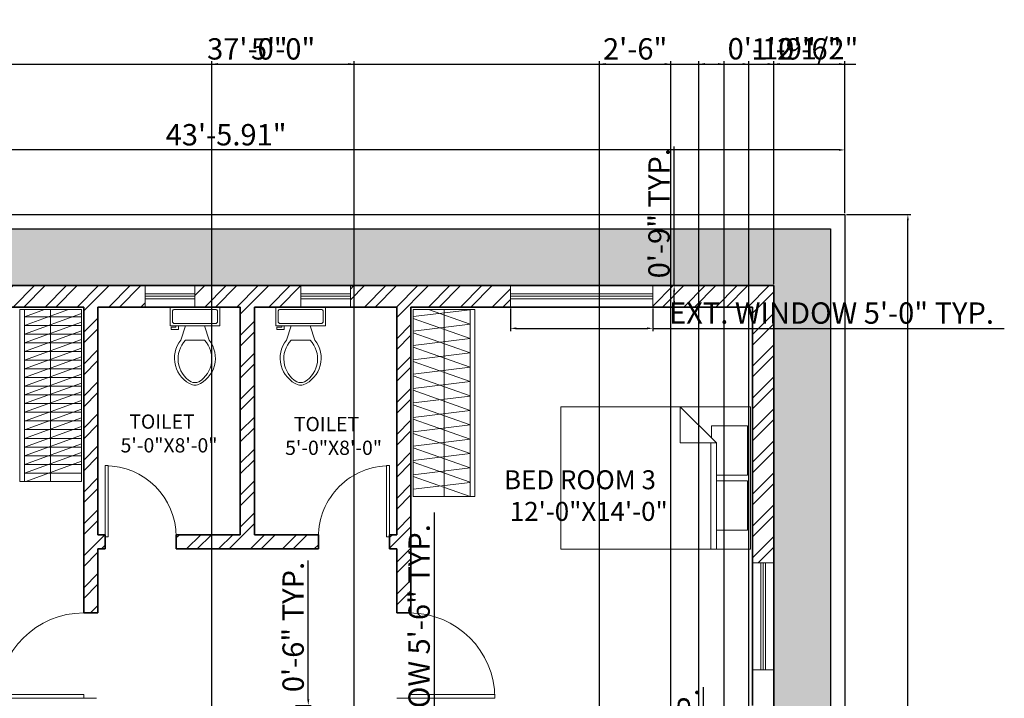
# Model space of a CAD drawing. Units: inches. Extents: x 108 to 883, y 608 to 1524.
# Tile 4 of 4: x 409 to 824, y 1238 to 1524. Entities that reach past the tile are written whole.
import ezdxf

# ---------------------------------------------------------------- set-up
doc = ezdxf.new("R2010")
doc.units = ezdxf.units.IN
for name, color, linetype, lineweight in [('A-ANNO-DIMS', 2, 'Continuous', 18), ('A-AREA-IDEN', 7, 'Continuous', 18), ('A-DOOR', 4, 'Continuous', 18), ('A-FLOR-CASE', 9, 'Continuous', 18), ('A-FLOR-CASE-PATT', 252, 'Continuous', 13), ('A-FLOR-FIXT', 9, 'Continuous', 18), ('A-FURN', 8, 'Continuous', 18), ('A-WALL', 7, 'Continuous', 35), ('A-WALL-PATT', 252, 'Continuous', 13), ('C-PROP', 7, 'Continuous', 25)]:
    doc.layers.add(name, color=color, linetype=linetype, lineweight=lineweight)
doc.layers.add('A-GLAZ', color=244, linetype='Continuous', lineweight=18, true_color=0x991b1e)
doc.layers.add('L-PLNT-PATT', color=116, linetype='Continuous', lineweight=13, true_color=0x136734)
doc.styles.get("Standard").update_dxf_attribs({"font": 'arial.ttf'})
doc.dimstyles.new('ISO-25', dxfattribs={"dimtxt": 9, "dimasz": 2.5, "dimexe": 1.25, "dimexo": 0.625, "dimtad": 1, "dimlunit": 3, "dimtxsty": 'Standard', "dimcen": 2.5, "dimadec": 0, "dimazin": 0, "dimtfac": 1, "dimtmove": 0, "dimatfit": 3, "dimfxl": 1, "dimarcsym": 0})

# ---------------------------------------------------------------- blocks, each defined once
blk = doc.blocks.new('*U3')
for p, q in [((-40, 0), (-40, 6)), ((0, 0), (0, 6))]:
    blk.add_line(p, q)
blk.add_lwpolyline([(0, 0), (0, -40), (-1.75, -40), (-1.75, 0)], close=True)
blk.add_arc((0, 0), 40, 180, 270)
blk = doc.blocks.new('*U4')
for p, q in [((0, 0), (0, -6)), ((-40, 0), (-40, -6))]:
    blk.add_line(p, q)
blk.add_lwpolyline([(0, 0), (0, 40), (-1.75, 40), (-1.75, 0)], close=True)
blk.add_arc((0, 0), 40, 90, 180)
blk = doc.blocks.new('*U5')
for p, q in [((0, 0), (0, 6)), ((40, 0), (40, 6))]:
    blk.add_line(p, q)
blk.add_lwpolyline([(0, 0), (0, -40), (1.75, -40), (1.75, 0)], close=True)
blk.add_arc((0, 0), 40, 270, 0)
blk = doc.blocks.new('*U9')
for p, q in [((9.5, -6), (9.5, -2)), ((-8, -8.5), (-8, -8)), ((-7, -8), (-7, -9.5)), ((-4, -8), (-6, -14)), ((4, -8), (6, -14)), ((-10, -8.5), (-8, -8.5)), ((-10, -9.5), (-10, -8.5)), ((-7, -9.5), (-10, -9.5)), ((4, -14), (-4, -14))]:
    blk.add_line(p, q)
blk.add_lwpolyline([(10.5, -8), (10.5, 0), (-10.5, 0), (-10.5, -8)], close=True)
for points in [[(-9.5, -2), (-9.5, -6)], [(8.5, -1), (-8.5, -1)], [(-8.5, -7), (8.5, -7)]]:
    blk.add_lwpolyline(points)
for centre, radius, start, end in [((-8.62, -1.88), 0.884, 81.8699, 188.1301), ((8.62, -1.88), 0.884, 351.8699, 98.1301), ((-8.62, -6.12), 0.884, 171.8699, 278.1301), ((8.62, -6.12), 0.884, 261.8699, 8.1301), ((3.52, -21.58), 12.17, 141.4691, 247.9714), ((4.2, -21.82), 11.33, 136.3677, 238.9468), ((-3.52, -21.58), 12.17, 292.0284, 38.5307), ((-4.2, -21.82), 11.33, 301.053, 43.6321), ((0, -27.88), 4, 245.7318, 294.2682), ((0, -29), 4, 254.8605, 285.1395)]:
    blk.add_arc(centre, radius, start, end)
blk = doc.blocks.new('Bed - Queen')
for p, q in [((0, -80.00003), (0, 0)), ((0, 0), (59.99999, 0)), ((59.99999, 0), (59.99999, -80.00003)), ((7.99999, -1.2), (28.79998, -1.2)), ((7.99999, -14.4), (7.99999, -1.2)), ((28.79998, -1.2), (28.79998, -14.4)), ((31.19999, -1.2), (51.99999, -1.2)), ((31.19999, -14.4), (31.19999, -1.2)), ((51.99999, -1.2), (51.99999, -16.4)), ((0, -14.4), (44.8, -14.4)), ((59.99999, -29.6), (44.8, -14.4)), ((44.8, -14.4), (44.8, -29.6)), ((51.99999, -16.4), (46.79936, -16.4)), ((44.8, -16.8), (0, -16.8)), ((44.8, -29.6), (59.99999, -29.6)), ((59.99999, -80.00003), (0, -80.00003))]:
    blk.add_line(p, q)
blk = doc.blocks.new('*D14')
at = {"layer": 'A-ANNO-DIMS', "color": 0, "lineweight": -2, "transparency": 16777216}
for p, q in [((757.75, 1442.18), (784.93, 1442.18)), ((783.68, 667.61), (783.68, 1439.68)), ((757.75, 665.11), (784.93, 665.11))]:
    blk.add_line(p, q, dxfattribs=at)
at = {"layer": 'A-ANNO-DIMS', "color": 0, "transparency": 16777216}
for points in [[(783.26, 1439.68), (784.09, 1439.68), (783.68, 1442.18)], [(783.26, 667.61), (784.09, 667.61), (783.68, 665.11)]]:
    blk.add_solid(points, dxfattribs=at)
at = {"layer": 'Defpoints', "color": 0, "transparency": 16777216}
for p in [(757.12, 1442.18), (783.68, 1442.18), (757.12, 665.11)]:
    blk.add_point(p, dxfattribs=at)
at = {"layer": 'A-ANNO-DIMS', "color": 0, "transparency": 16777216, "insert": (778.46, 1053.64), "char_height": 9, "attachment_point": 5, "rotation": 90}
blk.add_mtext('64\'-9.07"', dxfattribs=at)
blk = doc.blocks.new('*D15')
at = {"layer": 'A-ANNO-DIMS', "color": 0, "lineweight": -2, "transparency": 16777216}
for p, q in [((235.21, 1442.8), (235.21, 1470.67)), ((757.12, 1442.8), (757.12, 1470.67)), ((754.62, 1469.42), (237.71, 1469.42))]:
    blk.add_line(p, q, dxfattribs=at)
at = {"layer": 'A-ANNO-DIMS', "color": 0, "transparency": 16777216}
for points in [[(237.71, 1469.84), (237.71, 1469.01), (235.21, 1469.42)], [(754.62, 1469.84), (754.62, 1469.01), (757.12, 1469.42)]]:
    blk.add_solid(points, dxfattribs=at)
at = {"layer": 'Defpoints', "color": 0, "transparency": 16777216}
for p in [(235.21, 1469.42), (235.21, 1442.18), (757.12, 1442.18)]:
    blk.add_point(p, dxfattribs=at)
at = {"layer": 'A-ANNO-DIMS', "color": 0, "transparency": 16777216, "insert": (496.17, 1474.65), "char_height": 9, "attachment_point": 5}
blk.add_mtext('43\'-5.91"', dxfattribs=at)
blk = doc.blocks.new('WIN-45IN-EXT')
for p, q in [((3.5, 45), (3.5, 0)), ((4.5, 45), (4.5, 0)), ((5.5, 45), (5.5, 0))]:
    blk.add_line(p, q)
blk.add_lwpolyline([(9, 45), (9, 0), (0, 0), (0, 45)], close=True)
blk = doc.blocks.new('WIN-60IN-EXT')
for p, q in [((60, 5.5), (0, 5.5)), ((60, 4.5), (0, 4.5)), ((60, 3.5), (0, 3.5))]:
    blk.add_line(p, q)
blk.add_lwpolyline([(60, 9), (60, 0), (0, 0), (0, 9)], close=True)
blk = doc.blocks.new('WIN-21IN-EXT')
for p, q in [((0, 5.5), (21, 5.5)), ((0, 4.5), (21, 4.5)), ((0, 3.5), (21, 3.5))]:
    blk.add_line(p, q)
blk.add_lwpolyline([(0, 9), (21, 9), (21, 0), (0, 0)], close=True)
blk = doc.blocks.new('*D24')
at = {"layer": 'A-ANNO-DIMS', "color": 0, "lineweight": -2, "transparency": 16777216}
for p, q in [((616.12, 1402.55), (616.12, 1392.93)), ((676.12, 1402.55), (676.12, 1392.93)), ((618.62, 1394.18), (673.62, 1394.18)), ((676.12, 1394.18), (824.36, 1394.18))]:
    blk.add_line(p, q, dxfattribs=at)
at = {"layer": 'A-ANNO-DIMS', "color": 0, "transparency": 16777216}
for points in [[(618.62, 1394.59), (618.62, 1393.76), (616.12, 1394.18)], [(673.62, 1394.59), (673.62, 1393.76), (676.12, 1394.18)]]:
    blk.add_solid(points, dxfattribs=at)
at = {"layer": 'Defpoints', "color": 0, "transparency": 16777216}
for p in [(616.12, 1403.18), (676.12, 1403.18), (676.12, 1394.18)]:
    blk.add_point(p, dxfattribs=at)
at = {"layer": 'A-ANNO-DIMS', "color": 0, "transparency": 16777216, "insert": (751.49, 1399.46), "char_height": 9, "attachment_point": 5}
blk.add_mtext('EXT. WINDOW 5\'-0" TYP.', dxfattribs=at)
blk = doc.blocks.new('*D25')
at = {"layer": 'A-ANNO-DIMS', "color": 0, "lineweight": -2, "transparency": 16777216}
for p, q in [((685.12, 1412.18), (685.12, 1470.79)), ((676.75, 1412.18), (686.37, 1412.18)), ((685.12, 1405.68), (685.12, 1409.68)), ((676.75, 1403.18), (686.37, 1403.18))]:
    blk.add_line(p, q, dxfattribs=at)
at = {"layer": 'A-ANNO-DIMS', "color": 0, "transparency": 16777216}
for points in [[(684.7, 1409.68), (685.54, 1409.68), (685.12, 1412.18)], [(684.7, 1405.68), (685.54, 1405.68), (685.12, 1403.18)]]:
    blk.add_solid(points, dxfattribs=at)
at = {"layer": 'Defpoints', "color": 0, "transparency": 16777216}
for p in [(676.12, 1412.18), (685.12, 1412.18), (676.12, 1403.18)]:
    blk.add_point(p, dxfattribs=at)
at = {"layer": 'A-ANNO-DIMS', "color": 0, "transparency": 16777216, "insert": (679.9, 1442.73), "char_height": 9, "attachment_point": 5, "rotation": 90}
blk.add_mtext('0\'-9" TYP.', dxfattribs=at)
blk = doc.blocks.new('*D26')
at = {"layer": 'A-ANNO-DIMS', "color": 0, "lineweight": -2, "transparency": 16777216}
for p, q in [((484.83, 1228.55), (484.83, 1221.93)), ((524.83, 1228.55), (524.83, 1221.93)), ((487.33, 1223.18), (522.33, 1223.18)), ((524.83, 1223.18), (690.18, 1223.18))]:
    blk.add_line(p, q, dxfattribs=at)
at = {"layer": 'A-ANNO-DIMS', "color": 0, "transparency": 16777216}
for points in [[(487.33, 1223.59), (487.33, 1222.76), (484.83, 1223.18)], [(522.33, 1223.59), (522.33, 1222.76), (524.83, 1223.18)]]:
    blk.add_solid(points, dxfattribs=at)
at = {"layer": 'Defpoints', "color": 0, "transparency": 16777216}
for p in [(484.83, 1229.18), (524.83, 1229.18), (524.83, 1223.18)]:
    blk.add_point(p, dxfattribs=at)
at = {"layer": 'A-ANNO-DIMS', "color": 0, "transparency": 16777216, "insert": (608.75, 1228.46), "char_height": 9, "attachment_point": 5}
blk.add_mtext('COURT WINDOW 3\'-4" TYP.', dxfattribs=at)
blk = doc.blocks.new('*D27')
at = {"layer": 'A-ANNO-DIMS', "color": 0, "lineweight": -2, "transparency": 16777216}
for p, q in [((530.83, 1237.68), (530.83, 1296.29)), ((525.45, 1235.18), (532.08, 1235.18)), ((530.83, 1229.18), (530.83, 1235.18)), ((525.45, 1229.18), (532.08, 1229.18)), ((530.83, 1226.68), (530.83, 1224.18))]:
    blk.add_line(p, q, dxfattribs=at)
at = {"layer": 'A-ANNO-DIMS', "color": 0, "transparency": 16777216}
for points in [[(530.41, 1237.68), (531.24, 1237.68), (530.83, 1235.18)], [(530.41, 1226.68), (531.24, 1226.68), (530.83, 1229.18)]]:
    blk.add_solid(points, dxfattribs=at)
at = {"layer": 'Defpoints', "color": 0, "transparency": 16777216}
for p in [(524.83, 1235.18), (530.83, 1235.18), (524.83, 1229.18)]:
    blk.add_point(p, dxfattribs=at)
at = {"layer": 'A-ANNO-DIMS', "color": 0, "transparency": 16777216, "insert": (525.61, 1268.23), "char_height": 9, "attachment_point": 5, "rotation": 90}
blk.add_mtext('0\'-6" TYP.', dxfattribs=at)
blk = doc.blocks.new('*D32')
at = {"layer": 'A-ANNO-DIMS', "color": 0, "lineweight": -2, "transparency": 16777216}
for p, q in [((584.02, 1151.18), (584.02, 1316.53)), ((574.75, 1151.18), (585.27, 1151.18)), ((584.02, 1087.68), (584.02, 1148.68)), ((574.75, 1085.18), (585.27, 1085.18))]:
    blk.add_line(p, q, dxfattribs=at)
at = {"layer": 'A-ANNO-DIMS', "color": 0, "transparency": 16777216}
for points in [[(583.6, 1148.68), (584.44, 1148.68), (584.02, 1151.18)], [(583.6, 1087.68), (584.44, 1087.68), (584.02, 1085.18)]]:
    blk.add_solid(points, dxfattribs=at)
at = {"layer": 'Defpoints', "color": 0, "transparency": 16777216}
for p in [(574.12, 1151.18), (584.02, 1151.18), (574.12, 1085.18)]:
    blk.add_point(p, dxfattribs=at)
at = {"layer": 'A-ANNO-DIMS', "color": 0, "transparency": 16777216, "insert": (578.74, 1235.11), "char_height": 9, "attachment_point": 5, "rotation": 90}
blk.add_mtext('COURT WINDOW 5\'-6" TYP.', dxfattribs=at)
blk = doc.blocks.new('*D41')
at = {"layer": 'A-ANNO-DIMS', "color": 0, "lineweight": -2, "transparency": 16777216}
for p, q in [((697.44, 1163.25), (697.44, 1242.83)), ((697.44, 1159.24), (697.44, 1160.75)), ((697.84, 1160.75), (698.69, 1160.75)), ((697.84, 1159.24), (698.69, 1159.24)), ((697.44, 1156.74), (697.44, 1154.24))]:
    blk.add_line(p, q, dxfattribs=at)
at = {"layer": 'A-ANNO-DIMS', "color": 0, "transparency": 16777216}
for points in [[(697.02, 1163.25), (697.85, 1163.25), (697.44, 1160.75)], [(697.02, 1156.74), (697.85, 1156.74), (697.44, 1159.24)]]:
    blk.add_solid(points, dxfattribs=at)
at = {"layer": 'Defpoints', "color": 0, "transparency": 16777216}
for p in [(697.21, 1160.75), (697.21, 1159.24), (697.44, 1160.75)]:
    blk.add_point(p, dxfattribs=at)
at = {"layer": 'A-ANNO-DIMS', "color": 0, "transparency": 16777216, "insert": (692.16, 1204.29), "char_height": 9, "attachment_point": 5, "rotation": 90}
blk.add_mtext('0\'-1 1/2" TYP.', dxfattribs=at)
blk = doc.blocks.new('*D44')
at = {"layer": 'A-ANNO-DIMS', "color": 0, "lineweight": -2, "transparency": 16777216}
for p, q in [((283.12, 1412.8), (283.12, 1506.88)), ((285.62, 1505.63), (724.62, 1505.63)), ((727.12, 1412.8), (727.12, 1506.88))]:
    blk.add_line(p, q, dxfattribs=at)
at = {"layer": 'A-ANNO-DIMS', "color": 0, "transparency": 16777216}
for points in [[(285.62, 1506.04), (285.62, 1505.21), (283.12, 1505.63)], [(724.62, 1506.04), (724.62, 1505.21), (727.12, 1505.63)]]:
    blk.add_solid(points, dxfattribs=at)
at = {"layer": 'Defpoints', "color": 0, "transparency": 16777216}
for p in [(727.12, 1505.63), (283.12, 1412.18), (727.12, 1412.18)]:
    blk.add_point(p, dxfattribs=at)
at = {"layer": 'A-ANNO-DIMS', "color": 0, "transparency": 16777216, "insert": (505.12, 1510.85), "char_height": 9, "attachment_point": 5}
blk.add_mtext('37\'-0"', dxfattribs=at)
blk = doc.blocks.new('*D46')
at = {"layer": 'A-ANNO-DIMS', "color": 0, "lineweight": -2, "transparency": 16777216}
for p, q in [((727.12, 1412.8), (727.12, 1506.88)), ((729.62, 1505.63), (754.62, 1505.63)), ((757.12, 1442.8), (757.12, 1506.88))]:
    blk.add_line(p, q, dxfattribs=at)
at = {"layer": 'A-ANNO-DIMS', "color": 0, "transparency": 16777216}
for points in [[(729.62, 1506.04), (729.62, 1505.21), (727.12, 1505.63)], [(754.62, 1506.04), (754.62, 1505.21), (757.12, 1505.63)]]:
    blk.add_solid(points, dxfattribs=at)
at = {"layer": 'Defpoints', "color": 0, "transparency": 16777216}
for p in [(757.12, 1505.63), (757.12, 1442.18), (727.12, 1412.18)]:
    blk.add_point(p, dxfattribs=at)
at = {"layer": 'A-ANNO-DIMS', "color": 0, "transparency": 16777216, "insert": (742.12, 1510.85), "char_height": 9, "attachment_point": 5}
blk.add_mtext('2\'-6"', dxfattribs=at)
blk = doc.blocks.new('*D52')
at = {"layer": 'A-ANNO-DIMS', "color": 0, "lineweight": -2, "transparency": 16777216}
for p, q in [((653.67, 1031.8), (653.67, 1506.88)), ((656.17, 1505.63), (681.17, 1505.63)), ((683.67, 1031.8), (683.67, 1506.88))]:
    blk.add_line(p, q, dxfattribs=at)
at = {"layer": 'A-ANNO-DIMS', "color": 0, "transparency": 16777216}
for points in [[(656.17, 1506.04), (656.17, 1505.21), (653.67, 1505.63)], [(681.17, 1506.04), (681.17, 1505.21), (683.67, 1505.63)]]:
    blk.add_solid(points, dxfattribs=at)
at = {"layer": 'Defpoints', "color": 0, "transparency": 16777216}
for p in [(683.67, 1505.63), (653.67, 1031.18), (683.67, 1031.18)]:
    blk.add_point(p, dxfattribs=at)
at = {"layer": 'A-ANNO-DIMS', "color": 0, "transparency": 16777216, "insert": (668.67, 1510.85), "char_height": 9, "attachment_point": 5}
blk.add_mtext('2\'-6"', dxfattribs=at)
blk = doc.blocks.new('*D53')
at = {"layer": 'A-ANNO-DIMS', "color": 0, "lineweight": -2, "transparency": 16777216}
for p, q in [((490.21, 802.3), (490.21, 1506.88)), ((492.71, 1505.63), (547.71, 1505.63)), ((550.21, 802.3), (550.21, 1506.88))]:
    blk.add_line(p, q, dxfattribs=at)
at = {"layer": 'A-ANNO-DIMS', "color": 0, "transparency": 16777216}
for points in [[(492.71, 1506.04), (492.71, 1505.21), (490.21, 1505.63)], [(547.71, 1506.04), (547.71, 1505.21), (550.21, 1505.63)]]:
    blk.add_solid(points, dxfattribs=at)
at = {"layer": 'Defpoints', "color": 0, "transparency": 16777216}
for p in [(550.21, 1505.63), (490.21, 801.68), (550.21, 801.68)]:
    blk.add_point(p, dxfattribs=at)
at = {"layer": 'A-ANNO-DIMS', "color": 0, "transparency": 16777216, "insert": (520.21, 1510.85), "char_height": 9, "attachment_point": 5}
blk.add_mtext('5\'-0"', dxfattribs=at)
blk = doc.blocks.new('*D54')
at = {"layer": 'A-ANNO-DIMS', "color": 0, "lineweight": -2, "transparency": 16777216}
for p, q in [((695.57, 1170.85), (695.57, 1506.88)), ((698.07, 1505.63), (714.08, 1505.63)), ((716.58, 1170.85), (716.58, 1506.88)), ((716.58, 1505.63), (743.4, 1505.63))]:
    blk.add_line(p, q, dxfattribs=at)
at = {"layer": 'A-ANNO-DIMS', "color": 0, "transparency": 16777216}
for points in [[(698.07, 1506.04), (698.07, 1505.21), (695.57, 1505.63)], [(714.08, 1506.04), (714.08, 1505.21), (716.58, 1505.63)]]:
    blk.add_solid(points, dxfattribs=at)
at = {"layer": 'Defpoints', "color": 0, "transparency": 16777216}
for p in [(716.58, 1505.63), (695.57, 1170.23), (716.58, 1170.23)]:
    blk.add_point(p, dxfattribs=at)
at = {"layer": 'A-ANNO-DIMS', "color": 0, "transparency": 16777216, "insert": (731.24, 1510.85), "char_height": 9, "attachment_point": 5}
blk.add_mtext('1\'-9"', dxfattribs=at)
blk = doc.blocks.new('*D58')
at = {"layer": 'A-ANNO-DIMS', "color": 0, "lineweight": -2, "transparency": 16777216}
for p, q in [((695.57, 1170.85), (695.57, 1506.88)), ((698.07, 1505.63), (703.67, 1505.63)), ((706.17, 1159.85), (706.17, 1506.88)), ((706.17, 1505.63), (761.81, 1505.63))]:
    blk.add_line(p, q, dxfattribs=at)
at = {"layer": 'A-ANNO-DIMS', "color": 0, "transparency": 16777216}
for points in [[(698.07, 1506.04), (698.07, 1505.21), (695.57, 1505.63)], [(703.67, 1506.04), (703.67, 1505.21), (706.17, 1505.63)]]:
    blk.add_solid(points, dxfattribs=at)
at = {"layer": 'Defpoints', "color": 0, "transparency": 16777216}
for p in [(706.17, 1505.63), (695.57, 1170.23), (706.17, 1159.23)]:
    blk.add_point(p, dxfattribs=at)
at = {"layer": 'A-ANNO-DIMS', "color": 0, "transparency": 16777216, "insert": (735.24, 1510.91), "char_height": 9, "attachment_point": 5}
blk.add_mtext('0\'-10 1/2"', dxfattribs=at)

msp = doc.modelspace()

# ---------------------------------------------------------------- hatches: boundary and pattern name
at = {"layer": 'A-FLOR-CASE-PATT'}
h = msp.add_hatch(dxfattribs=at)
h.set_pattern_fill('ANSI31', color=256, scale=1.085896, angle=-25.10349, style=0)
h.paths.add_polyline_path([(411.121, 1329.629), (415.68, 1329.629), (435.121, 1336.665), (435.121, 1402.177), (415.599, 1402.177), (411.121, 1400.556)])
h = msp.add_hatch(dxfattribs=at)
h.set_pattern_fill('ANSI31', color=256, scale=1.15354, angle=-45, style=0)
h.paths.add_polyline_path([(435.121, 1331.648), (435.121, 1400.554), (411.121, 1400.554), (411.121, 1331.648)])
h = msp.add_hatch(dxfattribs=at)
h.set_pattern_fill('ANSI31', color=256, scale=1.801461, angle=115.6058, style=0)
h.paths.add_polyline_path([(591.37, 1323.234), (599.121, 1323.234), (599.121, 1398.668), (589.153, 1402.177), (575.121, 1402.177), (575.121, 1328.954)])
h = msp.add_hatch(dxfattribs=at)
h.set_pattern_fill('ANSI31', color=256, scale=1.89675, angle=-38.0207, style=0)
h.paths.add_polyline_path([(599.121, 1326.563), (599.121, 1402.177), (578.282, 1402.177), (575.121, 1401.79), (575.121, 1323.625)])
at = {"layer": 'A-WALL-PATT'}
h = msp.add_hatch(dxfattribs=at)
h.set_pattern_fill('ANSI32', color=256)
h.paths.add_polyline_path([(373.121, 1085.177), (292.121, 1085.177), (292.121, 1127.011), (283.121, 1127.011), (283.121, 1085.177), (235.212, 1085.177), (235.212, 1029.423), (244.212, 1029.423), (244.212, 1079.177), (373.121, 1079.177), (373.121, 1084.577)])
h.paths.add_polyline_path([(349.212, 911.177), (244.212, 911.177), (244.212, 969.423), (235.212, 969.423), (235.212, 776.177), (266.885, 776.177), (266.885, 785.177), (244.212, 785.177), (244.212, 905.177), (316.212, 905.177), (316.212, 902.177), (322.212, 902.177), (322.212, 905.177), (349.212, 905.177)])
h.paths.add_polyline_path([(484.212, 839.177), (473.778, 839.177), (473.778, 830.177), (478.212, 830.177), (478.212, 770.177), (484.212, 770.177), (484.212, 801.677), (490.212, 801.677), (490.212, 806.177), (490.212, 807.677), (484.212, 807.677)])
h.paths.add_polyline_path([(562.212, 830.177), (566.671, 830.177), (566.671, 839.177), (556.212, 839.177), (556.212, 807.677), (550.212, 807.677), (550.212, 806.177), (550.212, 801.677), (556.212, 801.677), (556.212, 770.177), (562.212, 770.177)])
h.paths.add_polyline_path([(622.212, 848.109), (613.212, 848.109), (613.212, 839.177), (611.671, 839.177), (611.671, 830.177), (622.212, 830.177)])
h.paths.add_polyline_path([(690.201, 911.177), (619.212, 911.177), (619.212, 1031.177), (653.667, 1031.177), (653.667, 1037.177), (613.212, 1037.177), (613.212, 893.109), (622.212, 893.109), (622.212, 902.177), (690.201, 902.177)])
h.paths.add_polyline_path([(727.121, 941.177), (718.121, 941.177), (718.121, 911.177), (711.201, 911.177), (711.201, 902.177), (727.121, 902.177)])
h.paths.add_polyline_path([(727.121, 1103.177), (718.121, 1103.177), (718.121, 1037.177), (683.667, 1037.177), (683.667, 1031.177), (718.121, 1031.177), (718.121, 1001.177), (727.121, 1001.177)])
h.paths.add_polyline_path([(727.121, 1412.177), (676.121, 1412.177), (676.121, 1403.177), (718.121, 1403.177), (718.121, 1295.236), (727.121, 1295.236)])
h.paths.add_polyline_path([(574.121, 1403.177), (616.121, 1403.177), (616.121, 1412.177), (548.621, 1412.177), (548.621, 1403.177), (568.121, 1403.177), (568.121, 1307.177), (565.121, 1307.177), (565.121, 1301.177), (568.121, 1301.177), (568.121, 1274.177), (574.121, 1274.177)])
h.paths.add_polyline_path([(508.121, 1403.177), (527.621, 1403.177), (527.621, 1412.177), (483.029, 1412.177), (483.029, 1403.177), (502.121, 1403.177), (502.121, 1307.177), (475.121, 1307.177), (475.121, 1301.177), (535.121, 1301.177), (535.121, 1307.177), (508.121, 1307.177)])
h.paths.add_polyline_path([(462.029, 1412.177), (394.121, 1412.177), (394.121, 1403.177), (436.121, 1403.177), (436.121, 1274.177), (442.121, 1274.177), (442.121, 1301.177), (445.121, 1301.177), (445.121, 1307.177), (442.121, 1307.177), (442.121, 1403.177), (462.029, 1403.177)])
h.paths.add_polyline_path([(334.121, 1412.177), (283.121, 1412.177), (283.121, 1288.13), (292.121, 1288.13), (292.121, 1403.177), (334.121, 1403.177)])
at = {"layer": 'L-PLNT-PATT'}
h = msp.add_hatch(dxfattribs=at)
h.set_pattern_fill('CROSS', color=256)
h.paths.add_polyline_path([(751.121, 1436.177), (241.212, 1436.177), (241.212, 1085.177), (283.121, 1085.177), (283.121, 1412.177), (727.121, 1412.177), (727.121, 902.177), (751.121, 902.177)])

# ---------------------------------------------------------------- linework, layer by layer
at = {"layer": 'A-FLOR-CASE'}
for p, q in [((409.121, 1402.177), (435.121, 1402.177)), ((409.121, 1402.177), (409.121, 1329.629)), ((411.121, 1402.177), (411.121, 1329.629)), ((422.121, 1402.177), (422.121, 1329.629)), ((435.121, 1402.177), (435.121, 1329.629)), ((575.121, 1402.177), (575.121, 1323.234)), ((575.121, 1402.177), (601.121, 1402.177)), ((588.121, 1402.177), (588.121, 1323.234)), ((599.121, 1402.177), (599.121, 1323.234)), ((601.121, 1402.177), (601.121, 1323.234)), ((435.121, 1329.629), (409.121, 1329.629)), ((575.121, 1323.234), (601.121, 1323.234))]:
    msp.add_line(p, q, dxfattribs=at)
at = {"layer": 'A-WALL'}
for p, q in [((283.121, 1412.177), (727.121, 1412.177)), ((727.121, 1412.177), (727.121, 902.177)), ((292.121, 1403.177), (436.121, 1403.177)), ((436.121, 1403.177), (436.121, 1274.177)), ((442.121, 1403.177), (442.121, 1307.177)), ((442.121, 1403.177), (502.121, 1403.177)), ((502.121, 1403.177), (502.121, 1307.177)), ((508.121, 1403.177), (508.121, 1307.177)), ((508.121, 1403.177), (568.121, 1403.177)), ((568.121, 1403.177), (568.121, 1307.177)), ((574.121, 1403.177), (574.121, 1274.177)), ((574.121, 1403.177), (718.121, 1403.177)), ((718.121, 1403.177), (718.121, 1235.177)), ((442.121, 1307.177), (445.121, 1307.177)), ((445.121, 1301.177), (445.121, 1307.177)), ((475.121, 1301.177), (475.121, 1307.177)), ((475.121, 1307.177), (502.121, 1307.177)), ((508.121, 1307.177), (535.121, 1307.177)), ((535.121, 1307.177), (535.121, 1301.177)), ((565.121, 1307.177), (565.121, 1301.177)), ((565.121, 1307.177), (568.121, 1307.177)), ((442.121, 1301.177), (445.121, 1301.177)), ((442.121, 1301.177), (442.121, 1274.177)), ((475.121, 1301.177), (535.121, 1301.177)), ((565.121, 1301.177), (568.121, 1301.177)), ((568.121, 1301.177), (568.121, 1274.177)), ((442.121, 1274.177), (436.121, 1274.177)), ((568.121, 1274.177), (574.121, 1274.177))]:
    msp.add_line(p, q, dxfattribs=at)
at = {"layer": 'C-PROP'}
for p, q in [((235.212, 1442.177), (757.121, 1442.177)), ((757.121, 1442.177), (757.121, 665.11)), ((241.212, 1436.177), (751.121, 1436.177)), ((751.121, 1436.177), (751.121, 671.11))]:
    msp.add_line(p, q, dxfattribs=at)

# ---------------------------------------------------------------- block references
at = {"layer": 'A-DOOR'}
for name, p, xscale, yscale, zscale, rotation in [('*U3', (445.122, 1306.277), 0.7499760613271671, 0.7499760613271671, 0.7499760613271671, 180), ('*U5', (565.121, 1306.277), 0.7499760613271671, 0.7499760613271671, 0.7499760613271671, 180), ('*U3', (436.121, 1238.177), 0.8999869424387545, 0.8999869424387545, 0.8999869424387545, 270), ('*U4', (573.521, 1238.177), 0.8999869424387545, 0.8999869424387545, 0.8999869424387545, 270)]:
    msp.add_blockref(name, p, dxfattribs=dict(at, xscale=xscale, yscale=yscale, zscale=zscale, rotation=rotation))
at = {"layer": 'A-FLOR-FIXT'}
for p in [(483.029, 1403.177), (527.621, 1403.177)]:
    msp.add_blockref('*U9', p, dxfattribs=at)
at = {"layer": 'A-FURN', "xscale": -1, "rotation": 270}
msp.add_blockref('Bed - Queen', (717.322, 1301.077), dxfattribs=at)
at = {"layer": 'A-GLAZ'}
for name, p in [('WIN-21IN-EXT', (462.029, 1403.177)), ('WIN-21IN-EXT', (527.622, 1403.177)), ('WIN-60IN-EXT', (616.121, 1403.177)), ('WIN-45IN-EXT', (718.122, 1250.236))]:
    msp.add_blockref(name, p, dxfattribs=at)

# ---------------------------------------------------------------- texts
at = {"layer": 'A-AREA-IDEN', "attachment_point": 1}
for s, width, insert, char_height in [('  TOILET \\P5\'-0"X8\'-0"', 38.89205, (451.676, 1357.849), 6), ('  TOILET \\P5\'-0"X8\'-0"', 38.89205, (521.064, 1356.814), 6), ('BED ROOM 3\\P 12\'-0"X14\'-0"', 70.1831, (613.397, 1334.334), 8)]:
    msp.add_mtext_dynamic_manual_height_columns(s, width=width, gutter_width=12.5, heights=[0], dxfattribs=dict(at, insert=insert, char_height=char_height))

# ---------------------------------------------------------------- dimensions: what is measured, and where the dimension line sits
at = {"layer": 'A-ANNO-DIMS'}
for base, p1, p2, override, picture, middle in [((706.173, 1505.627), (695.567, 1170.227), (706.173, 1159.227), {"dimdec": 1, "dimlfac": 1, "dimrnd": 0, "dimzin": 1, "dimdsep": 46, "dimlunit": 4, "dimfrac": 2}, '*D58', (735.242, 1510.905)), ((727.121, 1505.627), (283.121, 1412.177), (727.121, 1412.177), {"dimdec": 1, "dimlfac": 1, "dimrnd": 0, "dimzin": 1, "dimdsep": 46, "dimlunit": 4, "dimfrac": 2}, '*D44', (505.121, 1510.85)), ((550.212, 1505.627), (490.212, 801.677), (550.212, 801.677), {"dimdec": 1, "dimlfac": 1, "dimrnd": 0, "dimzin": 1, "dimdsep": 46, "dimlunit": 4, "dimfrac": 2}, '*D53', (520.212, 1510.847)), ((683.667, 1505.627), (653.667, 1031.177), (683.667, 1031.177), {"dimdec": 1, "dimlfac": 1, "dimrnd": 0, "dimzin": 1, "dimdsep": 46, "dimlunit": 4, "dimfrac": 2}, '*D52', (668.667, 1510.847)), ((716.576, 1505.627), (695.567, 1170.227), (716.576, 1170.227), {"dimdec": 1, "dimlfac": 1, "dimrnd": 0, "dimzin": 1, "dimdsep": 46, "dimlunit": 4, "dimfrac": 2}, '*D54', (731.239, 1510.847)), ((757.121, 1505.627), (727.121, 1412.177), (757.121, 1442.177), {"dimdec": 1, "dimlfac": 1, "dimrnd": 0, "dimzin": 1, "dimdsep": 46, "dimlunit": 4, "dimfrac": 2}, '*D46', (742.121, 1510.847)), ((235.212, 1469.422), (757.121, 1442.177), (235.212, 1442.177), {"dimclrd": 0, "dimclre": 0, "dimclrt": 0}, '*D15', (496.167, 1474.645))]:
    dim = msp.add_linear_dim(base=base, p1=p1, p2=p2, dimstyle='ISO-25', override=override, dxfattribs=at)
    dim.commit()
    dim.dimension.update_dxf_attribs({"geometry": picture, "text_midpoint": middle})
for base, p1, p2, text, picture, middle in [((685.121, 1412.177), (676.121, 1403.177), (676.121, 1412.177), '<> TYP.', '*D25', (679.901, 1442.732)), ((584.021, 1151.177), (574.121, 1085.177), (574.121, 1151.177), 'COURT WINDOW <> TYP.', '*D32', (578.74, 1235.105)), ((530.826, 1235.177), (524.826, 1229.177), (524.826, 1235.177), '<> TYP.', '*D27', (525.605, 1268.232)), ((697.438, 1160.751), (697.211, 1159.24), (697.211, 1160.751), '<> TYP.', '*D41', (692.159, 1204.291))]:
    dim = msp.add_linear_dim(base=base, p1=p1, p2=p2, angle=90, text=text, dimstyle='ISO-25', override={"dimdec": 1, "dimlfac": 1, "dimrnd": 0, "dimzin": 1, "dimdsep": 46, "dimlunit": 4, "dimfrac": 2}, dxfattribs=at)
    dim.commit()
    dim.dimension.update_dxf_attribs({"geometry": picture, "text_midpoint": middle})
dim = msp.add_linear_dim(base=(783.676, 1442.177), p1=(757.121, 665.11), p2=(757.121, 1442.177), angle=90, dimstyle='ISO-25', override={"dimclrd": 0, "dimclre": 0, "dimclrt": 0}, dxfattribs=at)
dim.commit()
dim.dimension.update_dxf_attribs({"geometry": '*D14', "text_midpoint": (778.456, 1053.644)})
for base, p1, p2, text, picture, middle in [((676.121, 1394.177), (616.121, 1403.177), (676.121, 1403.177), 'EXT. WINDOW <> TYP.', '*D24', (751.489, 1399.458)), ((524.826, 1223.177), (484.826, 1229.177), (524.826, 1229.177), 'COURT WINDOW <> TYP.', '*D26', (608.754, 1228.461))]:
    dim = msp.add_linear_dim(base=base, p1=p1, p2=p2, text=text, dimstyle='ISO-25', override={"dimdec": 1, "dimlfac": 1, "dimrnd": 0, "dimzin": 1, "dimdsep": 46, "dimlunit": 4, "dimfrac": 2}, dxfattribs=at)
    dim.commit()
    dim.dimension.update_dxf_attribs({"geometry": picture, "text_midpoint": middle})

doc.saveas('drawing.dxf')
